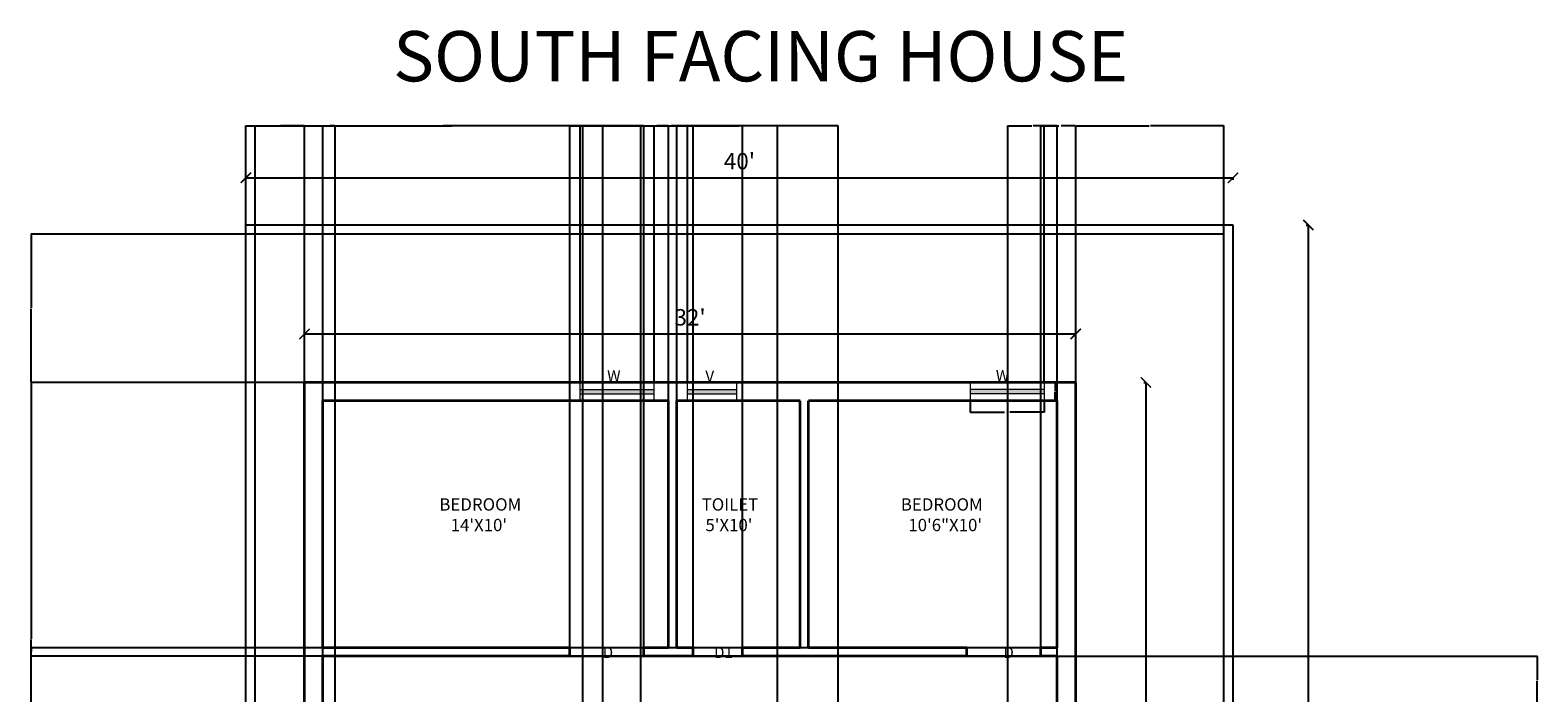
# Model space of a CAD drawing. Units: inches. Extents: x 502 to 1235, y -850 to 110.
# Tile 9 of 9: x 502 to 1235, y -212 to 110. Entities that reach past the tile are written whole.
import ezdxf

# ---------------------------------------------------------------- set-up
doc = ezdxf.new("R2010")
doc.units = ezdxf.units.IN
doc.header["$MEASUREMENT"] = 0
for name, color, linetype, lineweight in [('A-ANNO-DIMS', 2, 'Continuous', 18), ('A-ANNO-TEXT', 7, 'Continuous', 18), ('A-AREA-IDEN', 8, 'Continuous', 18), ('A-GLAZ-PATT', 5, 'Continuous', 13), ('C-PROP', 1, 'Continuous', 25), ('WALL', 1, 'Continuous', 35), ('WIN', 5, 'Continuous', 18)]:
    doc.layers.add(name, color=color, linetype=linetype, lineweight=lineweight)
doc.styles.get("Standard").update_dxf_attribs({"font": 'arial.ttf'})
doc.dimstyles.get("Standard").update_dxf_attribs({"dimtxt": 0.18, "dimasz": 0.18, "dimexe": 0.18, "dimexo": 0.0625, "dimgap": 0.09, "dimtad": 0, "dimtih": 1, "dimtoh": 1, "dimdec": 1, "dimzin": 0, "dimdsep": 46, "dimlunit": 4, "dimtxsty": 'Standard', "dimcen": 0.09, "dimadec": 0, "dimazin": 0, "dimtfac": 1, "dimtdec": 1, "dimtofl": 0, "dimtmove": 0, "dimatfit": 3, "dimfxl": 1, "dimtolj": 1, "dimtzin": 0, "dimarcsym": 0})

# ---------------------------------------------------------------- blocks, each defined once
blk = doc.blocks.new('_ArchTick')
at = {"color": 0, "linetype": 'ByBlock', "const_width": 0.15}
blk.add_lwpolyline([(-0.5, -0.5), (0.5, 0.5)], dxfattribs=at)
blk = doc.blocks.new('*D2')
at = {"layer": 'A-ANNO-DIMS', "color": 0, "lineweight": -2, "transparency": 16777216}
for p, q in [((606.89, 37.6), (606.89, 38.78)), ((606.89, 38.6), (1086.89, 38.6)), ((1086.89, 37.6), (1086.89, 38.78))]:
    blk.add_line(p, q, dxfattribs=at)
at = {"layer": 'Defpoints', "color": 0, "transparency": 16777216}
for p in [(1086.89, 38.6), (606.89, 15.65), (1086.89, 15.65)]:
    blk.add_point(p, dxfattribs=at)
at = {"layer": 'A-ANNO-DIMS', "color": 0, "lineweight": -2, "transparency": 16777216, "xscale": 5, "yscale": 5, "zscale": 5, "rotation": 180}
blk.add_blockref('_ArchTick', (606.89, 38.6), dxfattribs=at)
at = {"layer": 'A-ANNO-DIMS', "color": 0, "lineweight": -2, "transparency": 16777216, "xscale": 5, "yscale": 5, "zscale": 5}
blk.add_blockref('_ArchTick', (1086.89, 38.6), dxfattribs=at)
at = {"layer": 'A-ANNO-DIMS', "color": 0, "transparency": 16777216, "insert": (846.89, 46.68), "char_height": 8, "attachment_point": 5}
blk.add_mtext("\\A1;40'", dxfattribs=at)
blk = doc.blocks.new('*D3')
at = {"layer": 'A-ANNO-DIMS', "color": 0, "lineweight": -2, "transparency": 16777216}
for p, q in [((635.39, -38.3), (635.39, -37.12)), ((635.39, -37.3), (1010.39, -37.3)), ((1010.39, -38.3), (1010.39, -37.12))]:
    blk.add_line(p, q, dxfattribs=at)
at = {"layer": 'Defpoints', "color": 0, "transparency": 16777216}
for p in [(1010.39, -37.3), (635.39, -60.85), (1010.39, -60.85)]:
    blk.add_point(p, dxfattribs=at)
at = {"layer": 'A-ANNO-DIMS', "color": 0, "lineweight": -2, "transparency": 16777216, "xscale": 5, "yscale": 5, "zscale": 5, "rotation": 180}
blk.add_blockref('_ArchTick', (635.39, -37.3), dxfattribs=at)
at = {"layer": 'A-ANNO-DIMS', "color": 0, "lineweight": -2, "transparency": 16777216, "xscale": 5, "yscale": 5, "zscale": 5}
blk.add_blockref('_ArchTick', (1010.39, -37.3), dxfattribs=at)
at = {"layer": 'A-ANNO-DIMS', "color": 0, "transparency": 16777216, "insert": (822.89, -29.21), "char_height": 8, "attachment_point": 5}
blk.add_mtext("\\A1;32'", dxfattribs=at)
blk = doc.blocks.new('*D6')
at = {"layer": 'A-ANNO-DIMS', "color": 0, "lineweight": -2, "transparency": 16777216}
for p, q in [((1122.49, 15.65), (1123.67, 15.65)), ((1123.49, 15.65), (1123.49, -704.35)), ((1122.49, -704.35), (1123.67, -704.35))]:
    blk.add_line(p, q, dxfattribs=at)
at = {"layer": 'Defpoints', "color": 0, "transparency": 16777216}
for p in [(1086.89, 15.65), (1086.89, -704.35), (1123.49, -704.35)]:
    blk.add_point(p, dxfattribs=at)
at = {"layer": 'A-ANNO-DIMS', "color": 0, "lineweight": -2, "transparency": 16777216, "xscale": 5, "yscale": 5, "zscale": 5}
for p, rotation in [((1123.49, 15.65), 90), ((1123.49, -704.35), 270)]:
    blk.add_blockref('_ArchTick', p, dxfattribs=dict(at, rotation=rotation))
at = {"layer": 'A-ANNO-DIMS', "color": 0, "transparency": 16777216, "insert": (1115.41, -344.35), "char_height": 8, "attachment_point": 5, "rotation": 90}
blk.add_mtext("\\A1;60'", dxfattribs=at)
blk = doc.blocks.new('*D7')
at = {"layer": 'A-ANNO-DIMS', "color": 0, "lineweight": -2, "transparency": 16777216}
for p, q in [((1043.54, -60.85), (1044.72, -60.85)), ((1044.54, -60.85), (1044.54, -551.48)), ((1043.54, -551.48), (1044.72, -551.48))]:
    blk.add_line(p, q, dxfattribs=at)
at = {"layer": 'Defpoints', "color": 0, "transparency": 16777216}
for p in [(1010.39, -60.85), (1010.39, -551.48), (1044.54, -551.48)]:
    blk.add_point(p, dxfattribs=at)
at = {"layer": 'A-ANNO-DIMS', "color": 0, "lineweight": -2, "transparency": 16777216, "xscale": 5, "yscale": 5, "zscale": 5}
for p, rotation in [((1044.54, -60.85), 90), ((1044.54, -551.48), 270)]:
    blk.add_blockref('_ArchTick', p, dxfattribs=dict(at, rotation=rotation))
at = {"layer": 'A-ANNO-DIMS', "color": 0, "transparency": 16777216, "insert": (1036.52, -306.16), "char_height": 8, "attachment_point": 5, "rotation": 90}
blk.add_mtext("\\A1;42'", dxfattribs=at)
blk = doc.blocks.new('WIN-36IN')
for p, q in [((0, 0), (0, 9)), ((36, 0), (36, 9)), ((0, 5.5), (36, 5.5)), ((0, 3.5), (36, 3.5))]:
    blk.add_line(p, q)
blk = doc.blocks.new('VENT-24IN')
for p, q in [((0, 0), (0, 9)), ((24, 0), (24, 9)), ((0, 5.5), (24, 5.5)), ((0, 3.5), (24, 3.5))]:
    blk.add_line(p, q)
blk = doc.blocks.new('*D14')
at = {"layer": 'A-ANNO-DIMS', "color": 0, "lineweight": -2, "transparency": 16777216}
for p, q in [((959.07, -69.91), (959.07, -75.43)), ((995.07, -69.91), (995.07, -75.43)), ((959.25, -75.25), (975.84, -75.25)), ((994.89, -75.25), (978.3, -75.25))]:
    blk.add_line(p, q, dxfattribs=at)
at = {"layer": 'A-ANNO-DIMS', "color": 0, "transparency": 16777216}
for points in [[(959.25, -75.22), (959.25, -75.28), (959.07, -75.25)], [(994.89, -75.22), (994.89, -75.28), (995.07, -75.25)]]:
    blk.add_solid(points, dxfattribs=at)
at = {"layer": 'Defpoints', "color": 0, "transparency": 16777216}
for p in [(959.07, -69.85), (995.07, -69.85), (959.07, -75.25)]:
    blk.add_point(p, dxfattribs=at)
at = {"layer": 'A-ANNO-DIMS', "color": 0, "transparency": 16777216, "insert": (977.07, -75.25), "char_height": 0.18, "attachment_point": 5}
blk.add_mtext('\\A1;WINDOW 3\'-0" TYP.', dxfattribs=at)
blk = doc.blocks.new('*D15')
at = {"layer": 'A-ANNO-DIMS', "color": 0, "lineweight": -2, "transparency": 16777216}
for p, q in [((995.13, -60.85), (1000.65, -60.85)), ((1000.47, -61.03), (1000.47, -65.16)), ((1000.47, -69.67), (1000.47, -65.53)), ((995.13, -69.85), (1000.65, -69.85))]:
    blk.add_line(p, q, dxfattribs=at)
at = {"layer": 'A-ANNO-DIMS', "color": 0, "transparency": 16777216}
for points in [[(1000.44, -61.03), (1000.5, -61.03), (1000.47, -60.85)], [(1000.44, -69.67), (1000.5, -69.67), (1000.47, -69.85)]]:
    blk.add_solid(points, dxfattribs=at)
at = {"layer": 'Defpoints', "color": 0, "transparency": 16777216}
for p in [(995.07, -60.85), (995.07, -69.85), (1000.47, -69.85)]:
    blk.add_point(p, dxfattribs=at)
at = {"layer": 'A-ANNO-DIMS', "color": 0, "transparency": 16777216, "insert": (1000.47, -65.35), "char_height": 0.18, "attachment_point": 5}
blk.add_mtext('\\A1;0\'-9" TYP.', dxfattribs=at)
blk = doc.blocks.new('*D22')
at = {"layer": 'A-ANNO-DIMS', "color": 0, "lineweight": -2, "transparency": 16777216}
for p, q in [((611.39, 11.22), (611.39, 63.98)), ((611.57, 63.8), (623.06, 63.8)), ((635.21, 63.8), (623.72, 63.8)), ((635.39, -60.78), (635.39, 63.98))]:
    blk.add_line(p, q, dxfattribs=at)
at = {"layer": 'A-ANNO-DIMS', "color": 0, "transparency": 16777216}
for points in [[(611.57, 63.83), (611.57, 63.77), (611.39, 63.8)], [(635.21, 63.83), (635.21, 63.77), (635.39, 63.8)]]:
    blk.add_solid(points, dxfattribs=at)
at = {"layer": 'Defpoints', "color": 0, "transparency": 16777216}
for p in [(635.39, 63.8), (611.39, 11.15), (635.39, -60.85)]:
    blk.add_point(p, dxfattribs=at)
at = {"layer": 'A-ANNO-DIMS', "color": 0, "transparency": 16777216, "insert": (623.39, 63.8), "char_height": 0.18, "attachment_point": 5}
blk.add_mtext('\\A1;2\'-0"', dxfattribs=at)
blk = doc.blocks.new('*D23')
at = {"layer": 'A-ANNO-DIMS', "color": 0, "lineweight": -2, "transparency": 16777216}
for p, q in [((611.33, 11.15), (502.37, 11.15)), ((502.55, 10.97), (502.55, -24.66)), ((502.55, -60.67), (502.55, -25.03)), ((635.33, -60.85), (502.37, -60.85))]:
    blk.add_line(p, q, dxfattribs=at)
at = {"layer": 'A-ANNO-DIMS', "color": 0, "transparency": 16777216}
for points in [[(502.52, 10.97), (502.58, 10.97), (502.55, 11.15)], [(502.52, -60.67), (502.58, -60.67), (502.55, -60.85)]]:
    blk.add_solid(points, dxfattribs=at)
at = {"layer": 'Defpoints', "color": 0, "transparency": 16777216}
for p in [(611.39, 11.15), (502.55, -60.85), (635.39, -60.85)]:
    blk.add_point(p, dxfattribs=at)
at = {"layer": 'A-ANNO-DIMS', "color": 0, "transparency": 16777216, "insert": (502.55, -24.85), "char_height": 0.18, "attachment_point": 5}
blk.add_mtext('\\A1;6\'-0"', dxfattribs=at)
blk = doc.blocks.new('*D24')
at = {"layer": 'A-ANNO-DIMS', "color": 0, "lineweight": -2, "transparency": 16777216}
for p, q in [((1010.39, -60.78), (1010.39, 63.98)), ((1010.57, 63.8), (1046.06, 63.8)), ((1082.21, 63.8), (1046.72, 63.8)), ((1082.39, 11.22), (1082.39, 63.98))]:
    blk.add_line(p, q, dxfattribs=at)
at = {"layer": 'A-ANNO-DIMS', "color": 0, "transparency": 16777216}
for points in [[(1010.57, 63.83), (1010.57, 63.77), (1010.39, 63.8)], [(1082.21, 63.83), (1082.21, 63.77), (1082.39, 63.8)]]:
    blk.add_solid(points, dxfattribs=at)
at = {"layer": 'Defpoints', "color": 0, "transparency": 16777216}
for p in [(1082.39, 63.8), (1082.39, 11.15), (1010.39, -60.85)]:
    blk.add_point(p, dxfattribs=at)
at = {"layer": 'A-ANNO-DIMS', "color": 0, "transparency": 16777216, "insert": (1046.39, 63.8), "char_height": 0.18, "attachment_point": 5}
blk.add_mtext('\\A1;6\'-0"', dxfattribs=at)
blk = doc.blocks.new('*D25')
at = {"layer": 'A-ANNO-DIMS', "color": 0, "lineweight": -2, "transparency": 16777216}
for p, q in [((798.89, -699.78), (798.89, 63.98)), ((799.07, 63.8), (846.56, 63.8)), ((894.71, 63.8), (847.22, 63.8)), ((894.89, -699.78), (894.89, 63.98))]:
    blk.add_line(p, q, dxfattribs=at)
at = {"layer": 'A-ANNO-DIMS', "color": 0, "transparency": 16777216}
for points in [[(799.07, 63.83), (799.07, 63.77), (798.89, 63.8)], [(894.71, 63.83), (894.71, 63.77), (894.89, 63.8)]]:
    blk.add_solid(points, dxfattribs=at)
at = {"layer": 'Defpoints', "color": 0, "transparency": 16777216}
for p in [(894.89, 63.8), (798.89, -699.85), (894.89, -699.85)]:
    blk.add_point(p, dxfattribs=at)
at = {"layer": 'A-ANNO-DIMS', "color": 0, "transparency": 16777216, "insert": (846.89, 63.8), "char_height": 0.18, "attachment_point": 5}
blk.add_mtext('\\A1;8\'-0"', dxfattribs=at)
blk = doc.blocks.new('*D26')
at = {"layer": 'A-ANNO-DIMS', "color": 0, "lineweight": -2, "transparency": 16777216}
for p, q in [((606.89, -704.28), (606.89, 63.98)), ((607.07, 63.8), (702.5, 63.8)), ((798.71, 63.8), (703.28, 63.8)), ((798.89, -704.28), (798.89, 63.98))]:
    blk.add_line(p, q, dxfattribs=at)
at = {"layer": 'A-ANNO-DIMS', "color": 0, "transparency": 16777216}
for points in [[(607.07, 63.83), (607.07, 63.77), (606.89, 63.8)], [(798.71, 63.83), (798.71, 63.77), (798.89, 63.8)]]:
    blk.add_solid(points, dxfattribs=at)
at = {"layer": 'Defpoints', "color": 0, "transparency": 16777216}
for p in [(798.89, 63.8), (606.89, -704.35), (798.89, -704.35)]:
    blk.add_point(p, dxfattribs=at)
at = {"layer": 'A-ANNO-DIMS', "color": 0, "transparency": 16777216, "insert": (702.89, 63.8), "char_height": 0.18, "attachment_point": 5}
blk.add_mtext('\\A1;16\'-0"', dxfattribs=at)
blk = doc.blocks.new('*D27')
at = {"layer": 'A-ANNO-DIMS', "color": 0, "lineweight": -2, "transparency": 16777216}
for p, q in [((644.39, -217.78), (644.39, 63.98)), ((644.57, 63.8), (706.99, 63.8)), ((770.61, 63.8), (708.19, 63.8)), ((770.79, -217.78), (770.79, 63.98))]:
    blk.add_line(p, q, dxfattribs=at)
at = {"layer": 'A-ANNO-DIMS', "color": 0, "transparency": 16777216}
for points in [[(644.57, 63.83), (644.57, 63.77), (644.39, 63.8)], [(770.61, 63.83), (770.61, 63.77), (770.79, 63.8)]]:
    blk.add_solid(points, dxfattribs=at)
at = {"layer": 'Defpoints', "color": 0, "transparency": 16777216}
for p in [(770.79, 63.8), (644.39, -217.85), (770.79, -217.85)]:
    blk.add_point(p, dxfattribs=at)
at = {"layer": 'A-ANNO-DIMS', "color": 0, "transparency": 16777216, "insert": (707.59, 63.8), "char_height": 0.18, "attachment_point": 5}
blk.add_mtext('\\A1;10\'-6 1/2"', dxfattribs=at)
blk = doc.blocks.new('*D29')
at = {"layer": 'A-ANNO-DIMS', "color": 0, "lineweight": -2, "transparency": 16777216}
for p, q in [((644.45, -193.85), (1235.01, -193.85)), ((1234.83, -194.03), (1234.83, -205.66)), ((1234.83, -217.67), (1234.83, -206.03)), ((644.45, -217.85), (1235.01, -217.85))]:
    blk.add_line(p, q, dxfattribs=at)
at = {"layer": 'A-ANNO-DIMS', "color": 0, "transparency": 16777216}
for points in [[(1234.8, -194.03), (1234.86, -194.03), (1234.83, -193.85)], [(1234.8, -217.67), (1234.86, -217.67), (1234.83, -217.85)]]:
    blk.add_solid(points, dxfattribs=at)
at = {"layer": 'Defpoints', "color": 0, "transparency": 16777216}
for p in [(644.39, -193.85), (644.39, -217.85), (1234.83, -217.85)]:
    blk.add_point(p, dxfattribs=at)
at = {"layer": 'A-ANNO-DIMS', "color": 0, "transparency": 16777216, "insert": (1234.83, -205.85), "char_height": 0.18, "attachment_point": 5}
blk.add_mtext('\\A1;2\'-0"', dxfattribs=at)
blk = doc.blocks.new('*D33')
at = {"layer": 'A-ANNO-DIMS', "color": 0, "lineweight": -2, "transparency": 16777216}
for p, q in [((764.39, -189.78), (764.39, 63.98)), ((764.57, 63.8), (782.06, 63.8)), ((800.21, 63.8), (782.72, 63.8)), ((800.39, -189.78), (800.39, 63.98))]:
    blk.add_line(p, q, dxfattribs=at)
at = {"layer": 'A-ANNO-DIMS', "color": 0, "transparency": 16777216}
for points in [[(764.57, 63.83), (764.57, 63.77), (764.39, 63.8)], [(800.21, 63.83), (800.21, 63.77), (800.39, 63.8)]]:
    blk.add_solid(points, dxfattribs=at)
at = {"layer": 'Defpoints', "color": 0, "transparency": 16777216}
for p in [(800.39, 63.8), (764.39, -189.85), (800.39, -189.85)]:
    blk.add_point(p, dxfattribs=at)
at = {"layer": 'A-ANNO-DIMS', "color": 0, "transparency": 16777216, "insert": (782.39, 63.8), "char_height": 0.18, "attachment_point": 5}
blk.add_mtext('\\A1;3\'-0"', dxfattribs=at)
blk = doc.blocks.new('*D34')
at = {"layer": 'A-ANNO-DIMS', "color": 0, "lineweight": -2, "transparency": 16777216}
for p, q in [((800.39, -189.78), (800.39, 63.98)), ((800.57, 63.8), (806.07, 63.8)), ((812.21, 63.8), (806.71, 63.8)), ((812.39, -189.78), (812.39, 63.98))]:
    blk.add_line(p, q, dxfattribs=at)
at = {"layer": 'A-ANNO-DIMS', "color": 0, "transparency": 16777216}
for points in [[(800.57, 63.83), (800.57, 63.77), (800.39, 63.8)], [(812.21, 63.83), (812.21, 63.77), (812.39, 63.8)]]:
    blk.add_solid(points, dxfattribs=at)
at = {"layer": 'Defpoints', "color": 0, "transparency": 16777216}
for p in [(812.39, 63.8), (800.39, -189.85), (812.39, -189.85)]:
    blk.add_point(p, dxfattribs=at)
at = {"layer": 'A-ANNO-DIMS', "color": 0, "transparency": 16777216, "insert": (806.39, 63.8), "char_height": 0.18, "attachment_point": 5}
blk.add_mtext('\\A1;1\'-0"', dxfattribs=at)
blk = doc.blocks.new('*D35')
at = {"layer": 'A-ANNO-DIMS', "color": 0, "lineweight": -2, "transparency": 16777216}
for p, q in [((824.39, -189.78), (824.39, 63.98)), ((824.57, 63.8), (836.06, 63.8)), ((848.21, 63.8), (836.72, 63.8)), ((848.39, -189.78), (848.39, 63.98))]:
    blk.add_line(p, q, dxfattribs=at)
at = {"layer": 'A-ANNO-DIMS', "color": 0, "transparency": 16777216}
for points in [[(824.57, 63.83), (824.57, 63.77), (824.39, 63.8)], [(848.21, 63.83), (848.21, 63.77), (848.39, 63.8)]]:
    blk.add_solid(points, dxfattribs=at)
at = {"layer": 'Defpoints', "color": 0, "transparency": 16777216}
for p in [(848.39, 63.8), (824.39, -189.85), (848.39, -189.85)]:
    blk.add_point(p, dxfattribs=at)
at = {"layer": 'A-ANNO-DIMS', "color": 0, "transparency": 16777216, "insert": (836.39, 63.8), "char_height": 0.18, "attachment_point": 5}
blk.add_mtext('\\A1;2\'-0"', dxfattribs=at)
blk = doc.blocks.new('*D36')
at = {"layer": 'A-ANNO-DIMS', "color": 0, "lineweight": -2, "transparency": 16777216}
for p, q in [((816.39, -189.78), (816.39, 63.98)), ((816.57, 63.8), (820.06, 63.8)), ((824.21, 63.8), (820.72, 63.8)), ((824.39, -189.78), (824.39, 63.98))]:
    blk.add_line(p, q, dxfattribs=at)
at = {"layer": 'A-ANNO-DIMS', "color": 0, "transparency": 16777216}
for points in [[(816.57, 63.83), (816.57, 63.77), (816.39, 63.8)], [(824.21, 63.83), (824.21, 63.77), (824.39, 63.8)]]:
    blk.add_solid(points, dxfattribs=at)
at = {"layer": 'Defpoints', "color": 0, "transparency": 16777216}
for p in [(824.39, 63.8), (816.39, -189.85), (824.39, -189.85)]:
    blk.add_point(p, dxfattribs=at)
at = {"layer": 'A-ANNO-DIMS', "color": 0, "transparency": 16777216, "insert": (820.39, 63.8), "char_height": 0.18, "attachment_point": 5}
blk.add_mtext('\\A1;0\'-8"', dxfattribs=at)
blk = doc.blocks.new('*D37')
at = {"layer": 'A-ANNO-DIMS', "color": 0, "lineweight": -2, "transparency": 16777216}
for p, q in [((993.39, -189.78), (993.39, 63.98)), ((993.57, 63.8), (997.06, 63.8)), ((1001.21, 63.8), (997.72, 63.8)), ((1001.39, -189.78), (1001.39, 63.98))]:
    blk.add_line(p, q, dxfattribs=at)
at = {"layer": 'A-ANNO-DIMS', "color": 0, "transparency": 16777216}
for points in [[(993.57, 63.83), (993.57, 63.77), (993.39, 63.8)], [(1001.21, 63.83), (1001.21, 63.77), (1001.39, 63.8)]]:
    blk.add_solid(points, dxfattribs=at)
at = {"layer": 'Defpoints', "color": 0, "transparency": 16777216}
for p in [(1001.39, 63.8), (993.39, -189.85), (1001.39, -189.85)]:
    blk.add_point(p, dxfattribs=at)
at = {"layer": 'A-ANNO-DIMS', "color": 0, "transparency": 16777216, "insert": (997.39, 63.8), "char_height": 0.18, "attachment_point": 5}
blk.add_mtext('\\A1;0\'-8"', dxfattribs=at)
blk = doc.blocks.new('*D38')
at = {"layer": 'A-ANNO-DIMS', "color": 0, "lineweight": -2, "transparency": 16777216}
for p, q in [((993.33, -189.85), (502.37, -189.85)), ((502.55, -190.03), (502.55, -191.66)), ((993.33, -193.85), (502.37, -193.85)), ((502.55, -193.67), (502.55, -192.03))]:
    blk.add_line(p, q, dxfattribs=at)
at = {"layer": 'A-ANNO-DIMS', "color": 0, "transparency": 16777216}
for points in [[(502.52, -190.03), (502.58, -190.03), (502.55, -189.85)], [(502.52, -193.67), (502.58, -193.67), (502.55, -193.85)]]:
    blk.add_solid(points, dxfattribs=at)
at = {"layer": 'Defpoints', "color": 0, "transparency": 16777216}
for p in [(993.39, -189.85), (502.55, -193.85), (993.39, -193.85)]:
    blk.add_point(p, dxfattribs=at)
at = {"layer": 'A-ANNO-DIMS', "color": 0, "transparency": 16777216, "insert": (502.55, -191.85), "char_height": 0.18, "attachment_point": 5}
blk.add_mtext('\\A1;0\'-4"', dxfattribs=at)
blk = doc.blocks.new('*D39')
at = {"layer": 'A-ANNO-DIMS', "color": 0, "lineweight": -2, "transparency": 16777216}
for p, q in [((644.39, -346.28), (644.39, 63.98)), ((644.57, 63.8), (647.06, 63.8)), ((650.21, 63.8), (647.72, 63.8)), ((650.39, -346.28), (650.39, 63.98))]:
    blk.add_line(p, q, dxfattribs=at)
at = {"layer": 'A-ANNO-DIMS', "color": 0, "transparency": 16777216}
for points in [[(644.57, 63.83), (644.57, 63.77), (644.39, 63.8)], [(650.21, 63.83), (650.21, 63.77), (650.39, 63.8)]]:
    blk.add_solid(points, dxfattribs=at)
at = {"layer": 'Defpoints', "color": 0, "transparency": 16777216}
for p in [(650.39, 63.8), (644.39, -346.35), (650.39, -346.35)]:
    blk.add_point(p, dxfattribs=at)
at = {"layer": 'A-ANNO-DIMS', "color": 0, "transparency": 16777216, "insert": (647.39, 63.8), "char_height": 0.18, "attachment_point": 5}
blk.add_mtext('\\A1;0\'-6"', dxfattribs=at)
blk = doc.blocks.new('*D43')
at = {"layer": 'A-ANNO-DIMS', "color": 0, "lineweight": -2, "transparency": 16777216}
for p, q in [((977.39, -422.28), (977.39, 63.98)), ((977.57, 63.8), (989.06, 63.8)), ((1001.21, 63.8), (989.72, 63.8)), ((1001.39, -422.28), (1001.39, 63.98))]:
    blk.add_line(p, q, dxfattribs=at)
at = {"layer": 'A-ANNO-DIMS', "color": 0, "transparency": 16777216}
for points in [[(977.57, 63.83), (977.57, 63.77), (977.39, 63.8)], [(1001.21, 63.83), (1001.21, 63.77), (1001.39, 63.8)]]:
    blk.add_solid(points, dxfattribs=at)
at = {"layer": 'Defpoints', "color": 0, "transparency": 16777216}
for p in [(1001.39, 63.8), (977.39, -422.35), (1001.39, -422.35)]:
    blk.add_point(p, dxfattribs=at)
at = {"layer": 'A-ANNO-DIMS', "color": 0, "transparency": 16777216, "insert": (989.39, 63.8), "char_height": 0.18, "attachment_point": 5}
blk.add_mtext('\\A1;2\'-0"', dxfattribs=at)
blk = doc.blocks.new('*D44')
at = {"layer": 'A-ANNO-DIMS', "color": 0, "lineweight": -2, "transparency": 16777216}
for p, q in [((780.39, -542.28), (780.39, 63.98)), ((780.57, 63.8), (822.56, 63.8)), ((865.21, 63.8), (823.22, 63.8)), ((865.39, -542.28), (865.39, 63.98))]:
    blk.add_line(p, q, dxfattribs=at)
at = {"layer": 'A-ANNO-DIMS', "color": 0, "transparency": 16777216}
for points in [[(780.57, 63.83), (780.57, 63.77), (780.39, 63.8)], [(865.21, 63.83), (865.21, 63.77), (865.39, 63.8)]]:
    blk.add_solid(points, dxfattribs=at)
at = {"layer": 'Defpoints', "color": 0, "transparency": 16777216}
for p in [(865.39, 63.8), (780.39, -542.35), (865.39, -542.35)]:
    blk.add_point(p, dxfattribs=at)
at = {"layer": 'A-ANNO-DIMS', "color": 0, "transparency": 16777216, "insert": (822.89, 63.8), "char_height": 0.18, "attachment_point": 5}
blk.add_mtext('\\A1;7\'-1"', dxfattribs=at)
blk = doc.blocks.new('*D49')
at = {"layer": 'A-ANNO-DIMS', "color": 0, "lineweight": -2, "transparency": 16777216}
for p, q in [((635.39, -60.78), (635.39, 63.98)), ((635.57, 63.8), (702.06, 63.8)), ((769.32, 63.8), (702.84, 63.8)), ((769.5, -60.78), (769.5, 63.98))]:
    blk.add_line(p, q, dxfattribs=at)
at = {"layer": 'A-ANNO-DIMS', "color": 0, "transparency": 16777216}
for points in [[(635.57, 63.83), (635.57, 63.77), (635.39, 63.8)], [(769.32, 63.83), (769.32, 63.77), (769.5, 63.8)]]:
    blk.add_solid(points, dxfattribs=at)
at = {"layer": 'Defpoints', "color": 0, "transparency": 16777216}
for p in [(769.5, 63.8), (635.39, -60.85), (769.5, -60.85)]:
    blk.add_point(p, dxfattribs=at)
at = {"layer": 'A-ANNO-DIMS', "color": 0, "transparency": 16777216, "insert": (702.45, 63.8), "char_height": 0.18, "attachment_point": 5}
blk.add_mtext('\\A1;11\'-2"', dxfattribs=at)
blk = doc.blocks.new('*D50')
at = {"layer": 'A-ANNO-DIMS', "color": 0, "lineweight": -2, "transparency": 16777216}
for p, q in [((805.5, -60.78), (805.5, 63.98)), ((805.68, 63.8), (813.26, 63.8)), ((821.47, 63.8), (813.9, 63.8)), ((821.65, -60.78), (821.65, 63.98))]:
    blk.add_line(p, q, dxfattribs=at)
at = {"layer": 'A-ANNO-DIMS', "color": 0, "transparency": 16777216}
for points in [[(805.68, 63.83), (805.68, 63.77), (805.5, 63.8)], [(821.47, 63.83), (821.47, 63.77), (821.65, 63.8)]]:
    blk.add_solid(points, dxfattribs=at)
at = {"layer": 'Defpoints', "color": 0, "transparency": 16777216}
for p in [(821.65, 63.8), (805.5, -60.85), (821.65, -60.85)]:
    blk.add_point(p, dxfattribs=at)
at = {"layer": 'A-ANNO-DIMS', "color": 0, "transparency": 16777216, "insert": (813.58, 63.8), "char_height": 0.18, "attachment_point": 5}
blk.add_mtext('\\A1;1\'-4"', dxfattribs=at)
blk = doc.blocks.new('*D51')
at = {"layer": 'A-ANNO-DIMS', "color": 0, "lineweight": -2, "transparency": 16777216}
for p, q in [((995.07, -60.78), (995.07, 63.98)), ((995.25, 63.8), (1002.2, 63.8)), ((1010.21, 63.8), (1003.26, 63.8)), ((1010.39, -60.78), (1010.39, 63.98))]:
    blk.add_line(p, q, dxfattribs=at)
at = {"layer": 'A-ANNO-DIMS', "color": 0, "transparency": 16777216}
for points in [[(995.25, 63.83), (995.25, 63.77), (995.07, 63.8)], [(1010.21, 63.83), (1010.21, 63.77), (1010.39, 63.8)]]:
    blk.add_solid(points, dxfattribs=at)
at = {"layer": 'Defpoints', "color": 0, "transparency": 16777216}
for p in [(1010.39, 63.8), (995.07, -60.85), (1010.39, -60.85)]:
    blk.add_point(p, dxfattribs=at)
at = {"layer": 'A-ANNO-DIMS', "color": 0, "transparency": 16777216, "insert": (1002.73, 63.8), "char_height": 0.18, "attachment_point": 5}
blk.add_mtext('\\A1;1\'-3 1/2"', dxfattribs=at)
blk = doc.blocks.new('*D52')
at = {"layer": 'A-ANNO-DIMS', "color": 0, "lineweight": -2, "transparency": 16777216}
for p, q in [((635.33, -60.85), (502.37, -60.85)), ((502.55, -61.03), (502.55, -185.41)), ((502.55, -310.17), (502.55, -185.78)), ((635.33, -310.35), (502.37, -310.35))]:
    blk.add_line(p, q, dxfattribs=at)
at = {"layer": 'A-ANNO-DIMS', "color": 0, "transparency": 16777216}
for points in [[(502.52, -61.03), (502.58, -61.03), (502.55, -60.85)], [(502.52, -310.17), (502.58, -310.17), (502.55, -310.35)]]:
    blk.add_solid(points, dxfattribs=at)
at = {"layer": 'Defpoints', "color": 0, "transparency": 16777216}
for p in [(502.55, -60.85), (635.39, -60.85), (635.39, -310.35)]:
    blk.add_point(p, dxfattribs=at)
at = {"layer": 'A-ANNO-DIMS', "color": 0, "transparency": 16777216, "insert": (502.55, -185.6), "char_height": 0.18, "attachment_point": 5}
blk.add_mtext('\\A1;20\'-9 1/2"', dxfattribs=at)

msp = doc.modelspace()

# ---------------------------------------------------------------- hatches: boundary and pattern name
at = {"layer": 'A-GLAZ-PATT'}
h = msp.add_hatch(color=256, dxfattribs=at)
h.dxf.hatch_style = 1
h.paths.add_polyline_path([(769.5, -64.35), (769.5, -66.35), (805.5, -66.35), (805.5, -64.35)])
h.paths.add_polyline_path([(845.65, -64.35), (821.65, -64.35), (821.65, -66.35), (845.65, -66.35)])
h.paths.add_polyline_path([(995.07, -64.35), (959.07, -64.35), (959.07, -66.35), (995.07, -66.35)])
h.paths.add_polyline_path([(1006.89, -358.85), (1004.89, -358.85), (1004.89, -394.85), (1006.89, -394.85)])
h.paths.add_polyline_path([(1006.89, -435.74), (1004.89, -435.74), (1004.89, -471.74), (1006.89, -471.74)])
h.paths.add_polyline_path([(874.64, -545.85), (874.64, -547.85), (910.64, -547.85), (910.64, -545.85)])
h.paths.add_polyline_path([(640.89, -310.35), (638.89, -310.35), (638.89, -334.35), (640.89, -334.35)])
h.paths.add_polyline_path([(640.89, -358.06), (638.89, -358.06), (638.89, -394.06), (640.89, -394.06)])

# ---------------------------------------------------------------- linework, layer by layer
at = {"layer": 'C-PROP'}
for p, q in [((606.89, -704.35), (606.89, 15.65)), ((1086.89, 15.65), (606.89, 15.65)), ((1086.89, -704.35), (1086.89, 15.65)), ((1082.39, 11.15), (611.39, 11.15)), ((611.39, -699.85), (611.39, 11.15)), ((1082.39, -699.85), (1082.39, 11.15))]:
    msp.add_line(p, q, dxfattribs=at)
at = {"layer": 'WALL'}
for p, q in [((1010.39, -60.85), (635.39, -60.85)), ((635.39, -615.85), (635.39, -60.85)), ((1010.39, -615.85), (1010.39, -60.85)), ((812.39, -69.85), (644.39, -69.85)), ((644.39, -189.85), (644.39, -69.85)), ((812.39, -189.85), (812.39, -69.85)), ((816.39, -189.85), (816.39, -69.85)), ((876.39, -69.85), (816.39, -69.85)), ((876.39, -189.85), (876.39, -69.85)), ((1001.39, -69.85), (880.39, -69.85)), ((880.39, -189.85), (880.39, -69.85)), ((1001.39, -189.85), (1001.39, -69.85)), ((764.39, -189.85), (644.39, -189.85)), ((764.39, -193.85), (764.39, -189.85)), ((800.39, -193.85), (800.39, -189.85)), ((812.39, -189.85), (800.39, -189.85)), ((824.39, -189.85), (816.39, -189.85)), ((824.39, -193.85), (824.39, -189.85)), ((848.39, -193.85), (848.39, -189.85)), ((876.39, -189.85), (848.39, -189.85)), ((957.39, -189.85), (880.39, -189.85)), ((957.39, -193.85), (957.39, -189.85)), ((1001.39, -189.85), (993.39, -189.85)), ((993.39, -193.85), (993.39, -189.85)), ((764.39, -193.85), (644.39, -193.85)), ((644.39, -294.35), (644.39, -193.85)), ((824.39, -193.85), (800.39, -193.85)), ((957.39, -193.85), (848.39, -193.85)), ((1001.39, -193.85), (993.39, -193.85)), ((1001.39, -418.35), (1001.39, -193.85))]:
    msp.add_line(p, q, dxfattribs=at)

# ---------------------------------------------------------------- block references
at = {"layer": 'WIN'}
for name, p in [('WIN-36IN', (769.5, -69.85)), ('VENT-24IN', (821.65, -69.85))]:
    msp.add_blockref(name, p, dxfattribs=at)
at = {"layer": 'WIN', "rotation": 180}
msp.add_blockref('WIN-36IN', (995.07, -60.85), dxfattribs=at)

# ---------------------------------------------------------------- texts
at = {"layer": 'A-ANNO-TEXT'}
for s, height, p in [('W', 5.44, (782.55, -60.38)), ('V', 5.44, (830.32, -60.52)), ('W', 5.44, (971.57, -60.29)), ('D', 5.44, (780.37, -194.86)), ('D1', 5.444, (834.5, -194.86)), ('D', 5.44, (975.2, -194.86))]:
    msp.add_text(s, height=height, dxfattribs=at).set_placement(p)
at = {"layer": 'A-ANNO-TEXT', "insert": (678.52, 109.93), "char_height": 24.4528, "attachment_point": 1}
msp.add_mtext_dynamic_manual_height_columns('SOUTH FACING HOUSE', width=395.3147, gutter_width=4.08, heights=[0], dxfattribs=at)
at = {"layer": 'A-AREA-IDEN', "char_height": 6, "attachment_point": 1}
for s, width, insert in [("    BEDROOM\\P       14'X10'", 54.3765, (693.65, -117.17)), ("    TOILET\\P     5'X10'", 44.2747, (821.18, -117.17)), ('   BEDROOM\\P     10\'6"X10\'', 53.3957, (919.86, -117.17))]:
    msp.add_mtext_dynamic_manual_height_columns(s, width=width, gutter_width=1, heights=[0], dxfattribs=dict(at, insert=insert))

# ---------------------------------------------------------------- dimensions: what is measured, and where the dimension line sits
at = {"layer": 'A-ANNO-DIMS'}
for base, p1, p2, override, picture, middle in [((798.89, 63.8), (606.89, -704.35), (798.89, -704.35), {"dimdec": 1, "dimlfac": 1, "dimrnd": 0, "dimzin": 1, "dimdsep": 46, "dimlunit": 4, "dimfrac": 2}, '*D26', (702.89, 63.8)), ((635.39, 63.8), (611.39, 11.15), (635.39, -60.85), {"dimdec": 1, "dimlfac": 1, "dimrnd": 0, "dimzin": 1, "dimdsep": 46, "dimlunit": 4, "dimfrac": 2}, '*D22', (623.39, 63.8)), ((769.5, 63.8), (635.39, -60.85), (769.5, -60.85), {"dimdec": 1, "dimlfac": 1, "dimrnd": 0, "dimzin": 1, "dimdsep": 46, "dimlunit": 4, "dimfrac": 2}, '*D49', (702.45, 63.8)), ((770.79, 63.8), (644.39, -217.85), (770.79, -217.85), {"dimdec": 1, "dimlfac": 1, "dimrnd": 0, "dimzin": 1, "dimdsep": 46, "dimlunit": 4, "dimfrac": 2}, '*D27', (707.59, 63.8)), ((650.39, 63.8), (644.39, -346.35), (650.39, -346.35), {"dimdec": 1, "dimlfac": 1, "dimrnd": 0, "dimzin": 1, "dimdsep": 46, "dimlunit": 4, "dimfrac": 2}, '*D39', (647.39, 63.8)), ((800.39, 63.8), (764.39, -189.85), (800.39, -189.85), {"dimdec": 1, "dimlfac": 1, "dimrnd": 0, "dimzin": 1, "dimdsep": 46, "dimlunit": 4, "dimfrac": 2}, '*D33', (782.39, 63.8)), ((865.39, 63.8), (780.39, -542.35), (865.39, -542.35), {"dimdec": 1, "dimlfac": 1, "dimrnd": 0, "dimzin": 1, "dimdsep": 46, "dimlunit": 4, "dimfrac": 2}, '*D44', (822.89, 63.8)), ((894.89, 63.8), (798.89, -699.85), (894.89, -699.85), {"dimdec": 1, "dimlfac": 1, "dimrnd": 0, "dimzin": 1, "dimdsep": 46, "dimlunit": 4, "dimfrac": 2}, '*D25', (846.89, 63.8)), ((812.39, 63.8), (800.39, -189.85), (812.39, -189.85), {"dimdec": 1, "dimlfac": 1, "dimrnd": 0, "dimzin": 1, "dimdsep": 46, "dimlunit": 4, "dimfrac": 2}, '*D34', (806.39, 63.8)), ((821.6491, 63.8044), (805.5034, -60.8456), (821.6491, -60.8456), {"dimdec": 1, "dimlfac": 1, "dimrnd": 0, "dimzin": 1, "dimdsep": 46, "dimlunit": 4, "dimfrac": 2}, '*D50', (813.5763, 63.8044)), ((824.39, 63.8), (816.39, -189.85), (824.39, -189.85), {"dimdec": 1, "dimlfac": 1, "dimrnd": 0, "dimzin": 1, "dimdsep": 46, "dimlunit": 4, "dimfrac": 2}, '*D36', (820.39, 63.8)), ((848.39, 63.8), (824.39, -189.85), (848.39, -189.85), {"dimdec": 1, "dimlfac": 1, "dimrnd": 0, "dimzin": 1, "dimdsep": 46, "dimlunit": 4, "dimfrac": 2}, '*D35', (836.39, 63.8)), ((1001.39, 63.8), (977.39, -422.35), (1001.39, -422.35), {"dimdec": 1, "dimlfac": 1, "dimrnd": 0, "dimzin": 1, "dimdsep": 46, "dimlunit": 4, "dimfrac": 2}, '*D43', (989.39, 63.8)), ((1001.39, 63.8), (993.39, -189.85), (1001.39, -189.85), {"dimdec": 1, "dimlfac": 1, "dimrnd": 0, "dimzin": 1, "dimdsep": 46, "dimlunit": 4, "dimfrac": 2}, '*D37', (997.39, 63.8)), ((1010.39, 63.8), (995.07, -60.85), (1010.39, -60.85), {"dimdec": 1, "dimlfac": 1, "dimrnd": 0, "dimzin": 1, "dimdsep": 46, "dimlunit": 4, "dimfrac": 2}, '*D51', (1002.73, 63.8)), ((1082.39, 63.8), (1010.39, -60.85), (1082.39, 11.15), {"dimdec": 1, "dimlfac": 1, "dimrnd": 0, "dimzin": 1, "dimdsep": 46, "dimlunit": 4, "dimfrac": 2}, '*D24', (1046.39, 63.8)), ((1086.89, 38.6), (606.89, 15.65), (1086.89, 15.65), {"dimtxt": 8, "dimasz": 5, "dimgap": 4, "dimtad": 1, "dimblk1": 'ArchTick', "dimblk2": 'ArchTick', "dimsah": 1, "dimclrd": 0, "dimclre": 0, "dimclrt": 0, "dimfxlon": 1}, '*D2', (846.89, 46.68))]:
    dim = msp.add_linear_dim(base=base, p1=p1, p2=p2, dimstyle='Standard', override=override, dxfattribs=at)
    dim.commit()
    dim.dimension.update_dxf_attribs({"geometry": picture, "text_midpoint": middle})
for base, p1, p2, override, picture, middle in [((1123.49, -704.35), (1086.89, 15.65), (1086.89, -704.35), {"dimtxt": 8, "dimasz": 5, "dimgap": 4, "dimtad": 1, "dimtih": 0, "dimblk1": 'ArchTick', "dimblk2": 'ArchTick', "dimsah": 1, "dimclrd": 0, "dimclre": 0, "dimclrt": 0, "dimfxlon": 1}, '*D6', (1115.41, -344.35)), ((502.55, -60.85), (611.39, 11.15), (635.39, -60.85), {"dimdec": 1, "dimlfac": 1, "dimrnd": 0, "dimzin": 1, "dimdsep": 46, "dimlunit": 4, "dimfrac": 2}, '*D23', (502.55, -24.85)), ((502.55, -60.85), (635.39, -310.35), (635.39, -60.85), {"dimdec": 1, "dimlfac": 1, "dimrnd": 0, "dimzin": 1, "dimdsep": 46, "dimlunit": 4, "dimfrac": 2}, '*D52', (502.55, -185.6)), ((502.55, -193.85), (993.39, -189.85), (993.39, -193.85), {"dimdec": 1, "dimlfac": 1, "dimrnd": 0, "dimzin": 1, "dimdsep": 46, "dimlunit": 4, "dimfrac": 2}, '*D38', (502.55, -191.85)), ((1234.83, -217.85), (644.39, -193.85), (644.39, -217.85), {"dimdec": 1, "dimlfac": 1, "dimrnd": 0, "dimzin": 1, "dimdsep": 46, "dimlunit": 4, "dimfrac": 2}, '*D29', (1234.83, -205.85))]:
    dim = msp.add_linear_dim(base=base, p1=p1, p2=p2, angle=90, dimstyle='Standard', override=override, dxfattribs=at)
    dim.commit()
    dim.dimension.update_dxf_attribs({"geometry": picture, "text_midpoint": middle})
dim = msp.add_linear_dim(base=(1010.39, -37.3), p1=(635.39, -60.85), p2=(1010.39, -60.85), text="32'", dimstyle='Standard', override={"dimtxt": 8, "dimasz": 5, "dimgap": 4, "dimtad": 1, "dimblk1": 'ArchTick', "dimblk2": 'ArchTick', "dimsah": 1, "dimclrd": 0, "dimclre": 0, "dimclrt": 0, "dimfxlon": 1}, dxfattribs=at)
dim.commit()
dim.dimension.update_dxf_attribs({"geometry": '*D3', "text_midpoint": (822.89, -29.21)})
for base, p1, p2, angle, text, override, picture, middle in [((1044.54, -551.48), (1010.39, -60.85), (1010.39, -551.48), 90, "42'", {"dimtxt": 8, "dimasz": 5, "dimgap": 4, "dimtad": 1, "dimtih": 0, "dimblk1": 'ArchTick', "dimblk2": 'ArchTick', "dimsah": 1, "dimclrd": 0, "dimclre": 0, "dimclrt": 0, "dimfxlon": 1}, '*D7', (1036.52, -306.16)), ((1000.47, -69.85), (995.07, -60.85), (995.07, -69.85), 270, '<> TYP.', {"dimdec": 1, "dimlfac": 1, "dimrnd": 0, "dimzin": 1, "dimdsep": 46, "dimlunit": 4, "dimfrac": 2}, '*D15', (1000.47, -65.35)), ((959.07, -75.25), (995.07, -69.85), (959.07, -69.85), 180, 'WINDOW <> TYP.', {"dimdec": 1, "dimlfac": 1, "dimrnd": 0, "dimzin": 1, "dimdsep": 46, "dimlunit": 4, "dimfrac": 2}, '*D14', (977.07, -75.25))]:
    dim = msp.add_linear_dim(base=base, p1=p1, p2=p2, angle=angle, text=text, dimstyle='Standard', override=override, dxfattribs=at)
    dim.commit()
    dim.dimension.update_dxf_attribs({"geometry": picture, "text_midpoint": middle})

doc.saveas('drawing.dxf')
